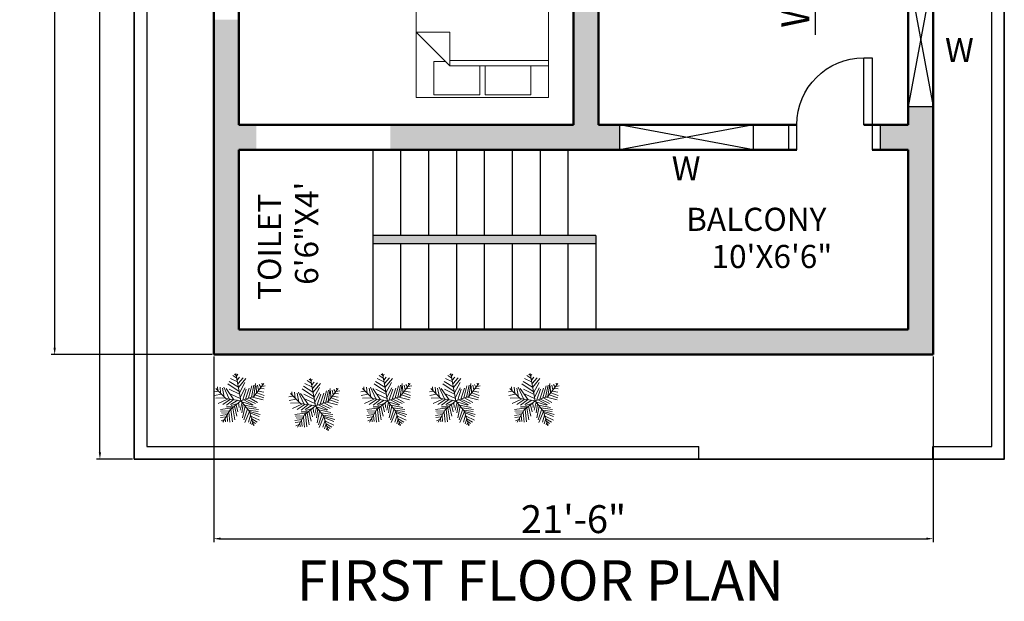
# Model space of a CAD drawing. Units: inches. Extents: x 2789 to 3623, y 2388 to 2993.
# Tile 3 of 5: x 3232 to 3586, y 2392 to 2601. Entities that reach past the tile are written whole.
import ezdxf

# ---------------------------------------------------------------- set-up
doc = ezdxf.new("R2010")
doc.units = ezdxf.units.IN
for name, color, linetype, lineweight in [('A-ANNO-DIMS', 2, 'Continuous', 18), ('A-ANNO-TEXT', 7, 'Continuous', 18), ('A-ANNO-TITL', 7, 'Continuous', 35), ('A-AREA-IDEN', 7, 'Continuous', 18), ('A-FLOR-STRS', 7, 'Continuous', 25), ('A-FURN', 8, 'Continuous', 18), ('A-WALL', 7, 'Continuous', 50), ('A-WALL-PATT', 5, 'Continuous', 13), ('C-PROP', 7, 'Continuous', 35), ('d', 1, 'Continuous', 25), ('L-PLNT', 94, 'Continuous', 13), ('L-WALL', 7, 'Continuous', 25), ('w', 170, 'Continuous', 25)]:
    doc.layers.add(name, color=color, linetype=linetype, lineweight=lineweight)
doc.styles.get("Standard").update_dxf_attribs({"font": 'arial.ttf'})
doc.dimstyles.new('ISO-25', dxfattribs={"dimtxt": 10, "dimasz": 2.5, "dimexe": 1.25, "dimexo": 0.625, "dimtad": 1, "dimlunit": 4, "dimtxsty": 'Standard', "dimcen": 2.5, "dimadec": 0, "dimazin": 0, "dimtfac": 1, "dimtmove": 0, "dimatfit": 3, "dimfxl": 1, "dimarcsym": 0})

# ---------------------------------------------------------------- blocks, each defined once
blk = doc.blocks.new('Bed - Queen')
for p, q in [((0, -80.00003), (0, 0)), ((0, 0), (59.99999, 0)), ((59.99999, 0), (59.99999, -80.00003)), ((7.99999, -1.2), (28.79998, -1.2)), ((7.99999, -14.4), (7.99999, -1.2)), ((28.79998, -1.2), (28.79998, -14.4)), ((31.19999, -1.2), (51.99999, -1.2)), ((31.19999, -14.4), (31.19999, -1.2)), ((51.99999, -1.2), (51.99999, -16.4)), ((0, -14.4), (44.8, -14.4)), ((44.8, -16.8), (0, -16.8)), ((59.99999, -29.6), (44.8, -14.4)), ((44.8, -14.4), (44.8, -29.6)), ((51.99999, -16.4), (46.79936, -16.4)), ((44.8, -29.6), (59.99999, -29.6)), ((59.99999, -80.00003), (0, -80.00003))]:
    blk.add_line(p, q)
blk = doc.blocks.new('*U11')
for p, q in [((-7.288, 39.707), (-21.778, 46.673)), ((-8.737, 47.138), (-17.069, 52.711)), ((-10.186, 53.64), (-13.084, 55.962)), ((0, 0), (-10.5, 57)), ((-9.099, 51.782), (-6.563, 55.962)), ((-7.65, 43.423), (-2.578, 49.46)), ((-5.839, 35.992), (4.667, 48.067)), ((-5.114, 27.632), (10.463, 46.673)), ((-31.5, 4.5), (-52.5, 25.5)), ((-48.585, 21.131), (-49.309, 29.026)), ((-43.513, 28.561), (-42.427, 15.558)), ((-38.442, 26.239), (-34.819, 7.663)), ((-35.544, 28.097), (-24.314, 3.947)), ((-14.533, 2.09), (-30.834, 25.31)), ((-3.665, 19.273), (-27.574, 35.527)), ((-5.114, 28.097), (-24.676, 40.636)), ((-24.314, 23.917), (-2.941, 13.7)), ((-2.941, 16.486), (8.652, 37.85)), ((-1.129, 6.734), (9.014, 26.704)), ((3.942, 1.625), (11.187, 24.381)), ((10.101, 3.483), (17.708, 26.239)), ((16.259, 5.805), (23.142, 31.348)), ((22.055, 7.198), (27.489, 32.277)), ((27, 9), (48, 36)), ((27.127, 9.056), (31.112, 35.992)), ((31.836, 30.883), (32.561, 16.486)), ((35.096, 32.741), (37.27, 22.524)), ((38.719, 34.134), (41.979, 28.561)), ((40.53, 25.775), (48.862, 24.846)), ((43.791, 29.954), (51.036, 30.883)), ((44.153, 36.456), (45.239, 32.741)), ((-47.498, 19.737), (-55.83, 18.344)), ((-40.615, 13.7), (-55.105, 10.913)), ((-33.37, 6.269), (-52.207, 5.34)), ((-28.299, 3.483), (-47.86, -5.805)), ((-21.416, 3.018), (-38.079, -8.128)), ((0, 0), (-31.5, 4.5)), ((-15.982, 2.09), (-30.11, -9.521)), ((0, 0), (-22.5, -19.5)), ((-6.563, 1.161), (-21.416, -8.128)), ((-20.691, 13.7), (-1.129, 4.876)), ((0, 0), (27, 9)), ((0, 0), (18, -22.5)), ((6.478, 1.625), (26.04, -8.592)), ((11.187, 3.483), (30.749, -5.805)), ((18.07, 5.805), (35.096, -3.483)), ((24.229, 7.663), (46.688, 1.625)), ((29.662, 12.307), (48.137, 6.269)), ((33.285, 16.486), (48.862, 10.913)), ((36.183, 19.737), (48.137, 17.88)), ((-17.431, -15.094), (-42.789, -18.809)), ((-22.5, -19.5), (-37.5, -45)), ((-15.257, -12.772), (-30.11, -12.772)), ((-20.691, -18.345), (-17.793, -44.352)), ((-6.563, -5.805), (-19.967, -9.985)), ((-17.069, -15.094), (-12.721, -40.172)), ((-13.446, -11.378), (-8.737, -32.741)), ((-9.461, -8.592), (-6.201, -23.453)), ((-4.752, -3.483), (-3.665, -14.629)), ((2.493, -3.019), (-1.491, -20.202)), ((1.769, -2.555), (24.229, -9.521)), ((5.029, -6.27), (2.131, -25.775)), ((9.014, -11.378), (3.58, -35.992)), ((14.085, -16.951), (6.478, -40.172)), ((7.565, -9.056), (32.198, -14.629)), ((12.274, -15.094), (36.907, -18.809)), ((16.259, -19.738), (36.183, -22.989)), ((-28.299, -29.026), (-42.789, -31.348)), ((-24.314, -21.596), (-42.427, -22.06)), ((-30.834, -34.135), (-42.427, -35.528)), ((-34.457, -39.708), (-40.978, -42.494)), ((-26.849, -26.24), (-40.253, -25.775)), ((-32.646, -36.921), (-31.921, -44.352)), ((-29.023, -30.884), (-27.936, -43.887)), ((-25.038, -23.918), (-22.865, -45.281)), ((18.07, -22.524), (8.289, -45.745)), ((20.244, -30.419), (15.897, -44.816)), ((18, -22.5), (27, -52.5)), ((18.433, -22.524), (40.53, -29.026)), ((19.157, -25.311), (38.719, -33.206)), ((22.78, -37.85), (19.519, -48.532)), ((21.331, -32.741), (39.081, -40.636)), ((22.78, -38.314), (34.372, -44.816)), ((24.591, -45.745), (23.142, -50.854)), ((24.591, -43.423), (30.749, -47.603)), ((26.764, -49.925), (28.213, -50.854))]:
    blk.add_line(p, q)
blk = doc.blocks.new('*D15')
at = {"layer": 'A-ANNO-DIMS', "color": 0, "lineweight": -2, "transparency": 16777216}
for p, q in [((3272.89, 2922.84), (3259.93, 2922.84)), ((3261.18, 2445.34), (3261.18, 2920.34)), ((3272.89, 2442.84), (3259.93, 2442.84))]:
    blk.add_line(p, q, dxfattribs=at)
at = {"layer": 'A-ANNO-DIMS', "color": 0, "transparency": 16777216}
for points in [[(3260.76, 2920.34), (3261.6, 2920.34), (3261.18, 2922.84)], [(3260.76, 2445.34), (3261.6, 2445.34), (3261.18, 2442.84)]]:
    blk.add_solid(points, dxfattribs=at)
at = {"layer": 'Defpoints', "color": 0, "transparency": 16777216}
for p in [(3261.18, 2922.84), (3273.51, 2922.84), (3273.51, 2442.84)]:
    blk.add_point(p, dxfattribs=at)
at = {"layer": 'A-ANNO-DIMS', "color": 0, "transparency": 16777216, "insert": (3255.45, 2682.84), "char_height": 10, "attachment_point": 5, "rotation": 90}
blk.add_mtext("40'", dxfattribs=at)
blk = doc.blocks.new('DOOR-24IN-JAMB-9IN')
for points in [[(0, 24), (-3, 24), (-3, 0), (0, 0)], [(-6, 0), (-3, 0), (-3, -9), (-6, -9)], [(24, 0), (27, 0), (27, -9), (24, -9)]]:
    blk.add_lwpolyline(points, close=True)
blk.add_arc((0, 0), 24, 0, 90)
blk = doc.blocks.new('WINDOW-48IN')
for p, q in [((48, 9), (0, 0)), ((48, 0), (0, 9))]:
    blk.add_line(p, q)
blk.add_lwpolyline([(0, 9), (0, 0), (48, 0), (48, 9)], close=True)
blk = doc.blocks.new('*D36')
at = {"layer": 'A-ANNO-DIMS', "color": 0, "lineweight": -2, "transparency": 16777216}
for p, q in [((3521.97, 2720.39), (3516.39, 2720.39)), ((3517.64, 2717.89), (3517.64, 2689.84)), ((3521.97, 2687.34), (3516.39, 2687.34)), ((3517.64, 2687.34), (3517.64, 2595.07))]:
    blk.add_line(p, q, dxfattribs=at)
at = {"layer": 'A-ANNO-DIMS', "color": 0, "transparency": 16777216}
for points in [[(3517.22, 2717.89), (3518.06, 2717.89), (3517.64, 2720.39)], [(3517.22, 2689.84), (3518.06, 2689.84), (3517.64, 2687.34)]]:
    blk.add_solid(points, dxfattribs=at)
at = {"layer": 'Defpoints', "color": 0, "transparency": 16777216}
for p in [(3522.6, 2720.39), (3517.64, 2687.34), (3522.6, 2687.34)]:
    blk.add_point(p, dxfattribs=at)
at = {"layer": 'A-ANNO-DIMS', "color": 0, "transparency": 16777216, "insert": (3511.84, 2639.96), "char_height": 10, "attachment_point": 5, "rotation": 90}
blk.add_mtext('WC 2\'-9" TYP.', dxfattribs=at)
blk = doc.blocks.new('*D44')
at = {"layer": 'A-ANNO-DIMS', "color": 0, "lineweight": -2, "transparency": 16777216}
for p, q in [((3302.01, 2479.72), (3302.01, 2413.04)), ((3560.01, 2479.72), (3560.01, 2413.04)), ((3304.51, 2414.29), (3557.51, 2414.29))]:
    blk.add_line(p, q, dxfattribs=at)
at = {"layer": 'A-ANNO-DIMS', "color": 0, "transparency": 16777216}
for points in [[(3304.51, 2414.71), (3304.51, 2413.88), (3302.01, 2414.29)], [(3557.51, 2414.71), (3557.51, 2413.88), (3560.01, 2414.29)]]:
    blk.add_solid(points, dxfattribs=at)
at = {"layer": 'Defpoints', "color": 0, "transparency": 16777216}
for p in [(3302.01, 2480.34), (3560.01, 2480.34), (3560.01, 2414.29)]:
    blk.add_point(p, dxfattribs=at)
at = {"layer": 'A-ANNO-DIMS', "color": 0, "transparency": 16777216, "insert": (3431.01, 2420.02), "char_height": 10, "attachment_point": 5}
blk.add_mtext('21\'-6"', dxfattribs=at)
blk = doc.blocks.new('*D45')
at = {"layer": 'A-ANNO-DIMS', "color": 0, "lineweight": -2, "transparency": 16777216}
for p, q in [((3301.39, 2894.34), (3243.71, 2894.34)), ((3244.96, 2482.84), (3244.96, 2891.84)), ((3301.39, 2480.34), (3243.71, 2480.34))]:
    blk.add_line(p, q, dxfattribs=at)
at = {"layer": 'A-ANNO-DIMS', "color": 0, "transparency": 16777216}
for points in [[(3244.55, 2891.84), (3245.38, 2891.84), (3244.96, 2894.34)], [(3244.55, 2482.84), (3245.38, 2482.84), (3244.96, 2480.34)]]:
    blk.add_solid(points, dxfattribs=at)
at = {"layer": 'Defpoints', "color": 0, "transparency": 16777216}
for p in [(3244.96, 2894.34), (3302.01, 2894.34), (3302.01, 2480.34)]:
    blk.add_point(p, dxfattribs=at)
at = {"layer": 'A-ANNO-DIMS', "color": 0, "transparency": 16777216, "insert": (3239.23, 2687.34), "char_height": 10, "attachment_point": 5, "rotation": 90}
blk.add_mtext('34\'-6"', dxfattribs=at)

msp = doc.modelspace()

# ---------------------------------------------------------------- hatches: boundary and pattern name
at = {"layer": 'A-WALL-PATT'}
h = msp.add_hatch(color=256, dxfattribs=at)
h.dxf.hatch_style = 1
h.paths.add_polyline_path([(3560.015, 2707.71), (3551.015, 2707.71), (3551.015, 2687.342), (3488.015, 2687.342), (3488.015, 2756.342), (3500.148, 2756.342), (3500.148, 2765.342), (3477.506, 2765.342), (3477.506, 2756.342), (3483.515, 2756.342), (3483.515, 2682.842), (3551.015, 2682.842), (3551.015, 2617.319), (3560.015, 2617.319)])
h.paths.add_polyline_path([(3560.015, 2817.229), (3551.015, 2817.229), (3551.015, 2812.239), (3551.015, 2765.342), (3533.148, 2765.342), (3533.148, 2756.342), (3551.015, 2756.342), (3551.015, 2731.71), (3560.015, 2731.71)])
h.paths.add_polyline_path([(3560.015, 2894.342), (3492.148, 2894.342), (3492.148, 2885.342), (3551.015, 2885.342), (3551.015, 2865.229), (3560.015, 2865.229)])
h.paths.add_polyline_path([(3444.148, 2894.342), (3363.151, 2894.342), (3363.151, 2885.342), (3431.015, 2885.342), (3431.015, 2765.342), (3368.943, 2765.342), (3368.943, 2756.342), (3444.506, 2756.342), (3444.506, 2765.342), (3440.015, 2765.342), (3440.015, 2885.342), (3444.148, 2885.342)])
h.paths.add_polyline_path([(3311.015, 2885.342), (3315.151, 2885.342), (3315.151, 2894.342), (3302.015, 2894.342), (3302.015, 2819.267), (3311.015, 2819.267)])
h.paths.add_polyline_path([(3311.015, 2756.342), (3332.943, 2756.342), (3332.943, 2765.342), (3311.015, 2765.342), (3311.015, 2771.267), (3302.015, 2771.267), (3302.015, 2648.516), (3311.015, 2648.516), (3311.015, 2682.842), (3320.883, 2682.842), (3320.883, 2687.342), (3311.015, 2687.342)])
h.paths.add_polyline_path([(3439.015, 2489.342), (3311.015, 2489.342), (3311.015, 2553.842), (3317.302, 2553.842), (3317.302, 2562.842), (3311.015, 2562.842), (3311.015, 2600.516), (3302.015, 2600.516), (3302.015, 2480.342), (3439.015, 2480.342)])
h.paths.add_polyline_path([(3447.515, 2562.842), (3440.015, 2562.842), (3440.015, 2687.342), (3353.883, 2687.342), (3353.883, 2682.842), (3431.015, 2682.842), (3431.015, 2562.842), (3365.302, 2562.842), (3365.302, 2553.842), (3447.515, 2553.842)])
h.paths.add_polyline_path([(3560.015, 2569.319), (3551.015, 2569.319), (3551.015, 2562.842), (3541.085, 2562.842), (3541.085, 2553.842), (3560.015, 2553.842)])
h.paths.add_polyline_path([(3439.015, 2523.092), (3359.015, 2523.092), (3359.015, 2520.092), (3439.015, 2520.092)], flags=17)
h.paths.add_polyline_path([(3341.726, 2503.274), (3341.726, 2543.14), (3329.011, 2543.14), (3329.011, 2503.274)], flags=25)
h.paths.add_polyline_path([(3328.42, 2497.829), (3328.42, 2542.718), (3315.535, 2542.718), (3315.535, 2497.829)], flags=25)
h.paths.add_polyline_path([(3476.819, 2492.441), (3529.584, 2492.441), (3529.584, 2505.156), (3476.819, 2505.156)], flags=9)
h.paths.add_polyline_path([(3482.427, 2505.748), (3529.241, 2505.748), (3529.241, 2518.633), (3482.427, 2518.633)], flags=9)
h.paths.add_polyline_path([(3491.312, 2778.023), (3533.511, 2778.023), (3533.511, 2790.738), (3491.312, 2790.738)], flags=9)
h.paths.add_polyline_path([(3467.584, 2791.33), (3549.839, 2791.33), (3549.839, 2804.214), (3467.584, 2804.214)], flags=9)
h.paths.add_polyline_path([(3489.974, 2712.567), (3519.954, 2712.567), (3519.954, 2720.13), (3489.974, 2720.13)], flags=25)
h.paths.add_polyline_path([(3493.529, 2720.481), (3522.128, 2720.481), (3522.128, 2728.14), (3493.529, 2728.14)], flags=25)
h.paths.add_polyline_path([(3443.312, 2609.496), (3485.511, 2609.496), (3485.511, 2622.211), (3443.312, 2622.211)], flags=9)
h.paths.add_polyline_path([(3444.938, 2623.016), (3478.097, 2623.016), (3478.097, 2635.468), (3444.938, 2635.468)], flags=9)
h.paths.add_polyline_path([(3353.282, 2645.374), (3395.481, 2645.374), (3395.481, 2658.089), (3353.282, 2658.089)], flags=9)
h.paths.add_polyline_path([(3347.837, 2658.68), (3428.155, 2658.68), (3428.155, 2671.565), (3347.837, 2671.565)], flags=9)
h.paths.add_polyline_path([(3345.461, 2717.778), (3391.776, 2717.778), (3391.776, 2730.493), (3345.461, 2730.493)], flags=9)
h.paths.add_polyline_path([(3340.017, 2731.086), (3399.739, 2731.086), (3399.739, 2743.962), (3340.017, 2743.962)], flags=9)
h.paths.add_polyline_path([(3345.461, 2806.621), (3387.66, 2806.621), (3387.66, 2819.336), (3345.461, 2819.336)], flags=9)
h.paths.add_polyline_path([(3340.017, 2819.929), (3398.431, 2819.929), (3398.431, 2832.806), (3340.017, 2832.806)], flags=9)
h = msp.add_hatch(color=256, dxfattribs=at)
h.dxf.hatch_style = 1
h.paths.add_polyline_path([(3560.015, 2569.319), (3551.015, 2569.319), (3551.015, 2562.842), (3541.085, 2562.842), (3541.085, 2553.842), (3551.015, 2553.842), (3551.015, 2489.342), (3311.015, 2489.342), (3311.015, 2553.842), (3317.302, 2553.842), (3317.302, 2562.842), (3311.015, 2562.842), (3311.015, 2600.516), (3302.015, 2600.516), (3302.015, 2480.342), (3560.015, 2480.342)])

# ---------------------------------------------------------------- linework, layer by layer
at = {"layer": 'A-FLOR-STRS'}
for p, q in [((3359.015, 2553.842), (3359.015, 2489.342)), ((3369.015, 2553.842), (3369.015, 2523.092)), ((3379.015, 2553.842), (3379.015, 2523.092)), ((3389.015, 2553.842), (3389.015, 2523.092)), ((3399.015, 2553.842), (3399.015, 2523.092)), ((3409.015, 2553.842), (3409.015, 2523.092)), ((3419.015, 2553.842), (3419.015, 2523.092)), ((3429.015, 2553.842), (3429.015, 2523.092)), ((3439.015, 2523.092), (3359.015, 2523.092)), ((3439.015, 2523.092), (3439.015, 2489.342)), ((3439.015, 2520.092), (3359.015, 2520.092)), ((3369.015, 2520.092), (3369.015, 2489.342)), ((3379.015, 2520.092), (3379.015, 2489.342)), ((3389.015, 2520.092), (3389.015, 2489.342)), ((3399.015, 2520.092), (3399.015, 2489.342)), ((3409.015, 2520.092), (3409.015, 2489.342)), ((3419.015, 2520.092), (3419.015, 2489.342)), ((3429.015, 2520.092), (3429.015, 2489.342))]:
    msp.add_line(p, q, dxfattribs=at)
at = {"layer": 'A-WALL'}
for p, q in [((3302.015, 2894.342), (3302.015, 2480.342)), ((3560.015, 2480.342), (3560.015, 2894.342)), ((3440.015, 2687.342), (3440.015, 2562.842)), ((3311.015, 2682.842), (3311.015, 2562.842)), ((3431.015, 2682.842), (3431.015, 2562.842)), ((3551.015, 2562.842), (3551.015, 2682.842)), ((3431.015, 2562.842), (3311.015, 2562.842)), ((3511.085, 2562.842), (3440.015, 2562.842)), ((3551.015, 2562.842), (3535.085, 2562.842)), ((3551.015, 2562.842), (3535.085, 2562.842)), ((3511.085, 2553.842), (3311.015, 2553.842)), ((3311.015, 2553.842), (3311.015, 2489.342)), ((3551.015, 2553.842), (3538.085, 2553.842)), ((3551.015, 2553.842), (3538.085, 2553.842)), ((3551.015, 2489.342), (3551.015, 2553.842)), ((3311.015, 2489.342), (3551.015, 2489.342)), ((3302.015, 2480.342), (3560.015, 2480.342))]:
    msp.add_line(p, q, dxfattribs=at)
at = {"layer": 'C-PROP'}
msp.add_lwpolyline([(3273.515, 2442.842), (3585.515, 2442.842), (3585.515, 2922.842), (3273.515, 2922.842)], close=True, dxfattribs=at)
at = {"layer": 'L-WALL'}
for p, q in [((3278.015, 2918.342), (3278.015, 2447.342)), ((3581.015, 2447.342), (3581.015, 2918.342)), ((3278.015, 2447.342), (3475.926, 2447.342)), ((3475.926, 2442.842), (3475.926, 2447.342)), ((3559.926, 2442.842), (3559.926, 2447.342)), ((3559.926, 2447.342), (3581.015, 2447.342))]:
    msp.add_line(p, q, dxfattribs=at)

# ---------------------------------------------------------------- block references
at = {"layer": 'A-FURN', "xscale": 0.7903362398625325, "yscale": 0.7903362398625325, "zscale": 0.7903362398625325, "rotation": 180}
msp.add_blockref('Bed - Queen', (3422.073, 2572.602), dxfattribs=at)
at = {"layer": 'd', "extrusion": (0, 0, -1), "zscale": -1}
msp.add_blockref('DOOR-24IN-JAMB-9IN', (-3535.085, 2562.842), dxfattribs=at)
at = {"layer": 'L-PLNT', "xscale": 0.1708886841943753, "yscale": 0.1708886841943753, "zscale": 0.1708886841943753}
for p in [(3311.72, 2463.813), (3338.446, 2462.027), (3364.275, 2463.813), (3388.87, 2463.813), (3417.218, 2463.813)]:
    msp.add_blockref('*U11', p, dxfattribs=at)
at = {"layer": 'w', "rotation": 90.00000000000207}
msp.add_blockref('WINDOW-48IN', (3560.014, 2569.319), dxfattribs=at)
at = {"layer": 'w'}
msp.add_blockref('WINDOW-48IN', (3447.514, 2553.842), dxfattribs=at)

# ---------------------------------------------------------------- texts
at = {"layer": 'A-ANNO-TEXT'}
for p in [(3564.263, 2585.302), (3466.255, 2542.832)]:
    msp.add_text('W', height=8.603, dxfattribs=at).set_placement(p)
at = {"layer": 'A-ANNO-TITL'}
msp.add_text('FIRST FLOOR PLAN ', height=14.48136, dxfattribs=at).set_placement((3331.798, 2392.088))
at = {"layer": 'A-AREA-IDEN'}
for s, p in [('6\'6"X4\'', (3339.466, 2505.393)), ('TOILET', (3326.131, 2499.976))]:
    msp.add_text(s, height=8.3011, rotation=90, dxfattribs=at).set_placement(p)
for s, p in [('BALCONY', (3471.414, 2524.734)), ('10\'X6\'6"', (3480.524, 2511.399))]:
    msp.add_text(s, height=8.3011, dxfattribs=at).set_placement(p)

# ---------------------------------------------------------------- dimensions: what is measured, and where the dimension line sits
at = {"layer": 'A-ANNO-DIMS'}
for base, p1, p2, override, picture, middle in [((3261.179, 2922.842), (3273.515, 2442.842), (3273.515, 2922.842), {"dimclrd": 0, "dimclre": 0, "dimclrt": 0}, '*D15', (3255.448, 2682.842)), ((3244.965, 2894.342), (3302.015, 2480.342), (3302.015, 2894.342), {"dimdec": 1, "dimlfac": 1, "dimrnd": 0, "dimzin": 1, "dimdsep": 46, "dimlunit": 4, "dimfrac": 2}, '*D45', (3239.23, 2687.342))]:
    dim = msp.add_linear_dim(base=base, p1=p1, p2=p2, angle=90, dimstyle='ISO-25', override=override, dxfattribs=at)
    dim.commit()
    dim.dimension.update_dxf_attribs({"geometry": picture, "text_midpoint": middle})
dim = msp.add_linear_dim(base=(3517.639, 2687.342), p1=(3522.596, 2720.388), p2=(3522.596, 2687.342), angle=270, text='WC <> TYP.', dimstyle='ISO-25', override={"dimdec": 1, "dimlfac": 1, "dimrnd": 0, "dimzin": 1, "dimdsep": 46, "dimlunit": 4, "dimfrac": 2}, dxfattribs=at)
dim.commit()
dim.dimension.update_dxf_attribs({"geometry": '*D36', "text_midpoint": (3511.844, 2639.957)})
dim = msp.add_linear_dim(base=(3560.015, 2414.292), p1=(3302.015, 2480.342), p2=(3560.015, 2480.342), dimstyle='ISO-25', override={"dimdec": 1, "dimlfac": 1, "dimrnd": 0, "dimzin": 1, "dimdsep": 46, "dimlunit": 4, "dimfrac": 2}, dxfattribs=at)
dim.commit()
dim.dimension.update_dxf_attribs({"geometry": '*D44', "text_midpoint": (3431.015, 2420.022)})

doc.saveas('drawing.dxf')
